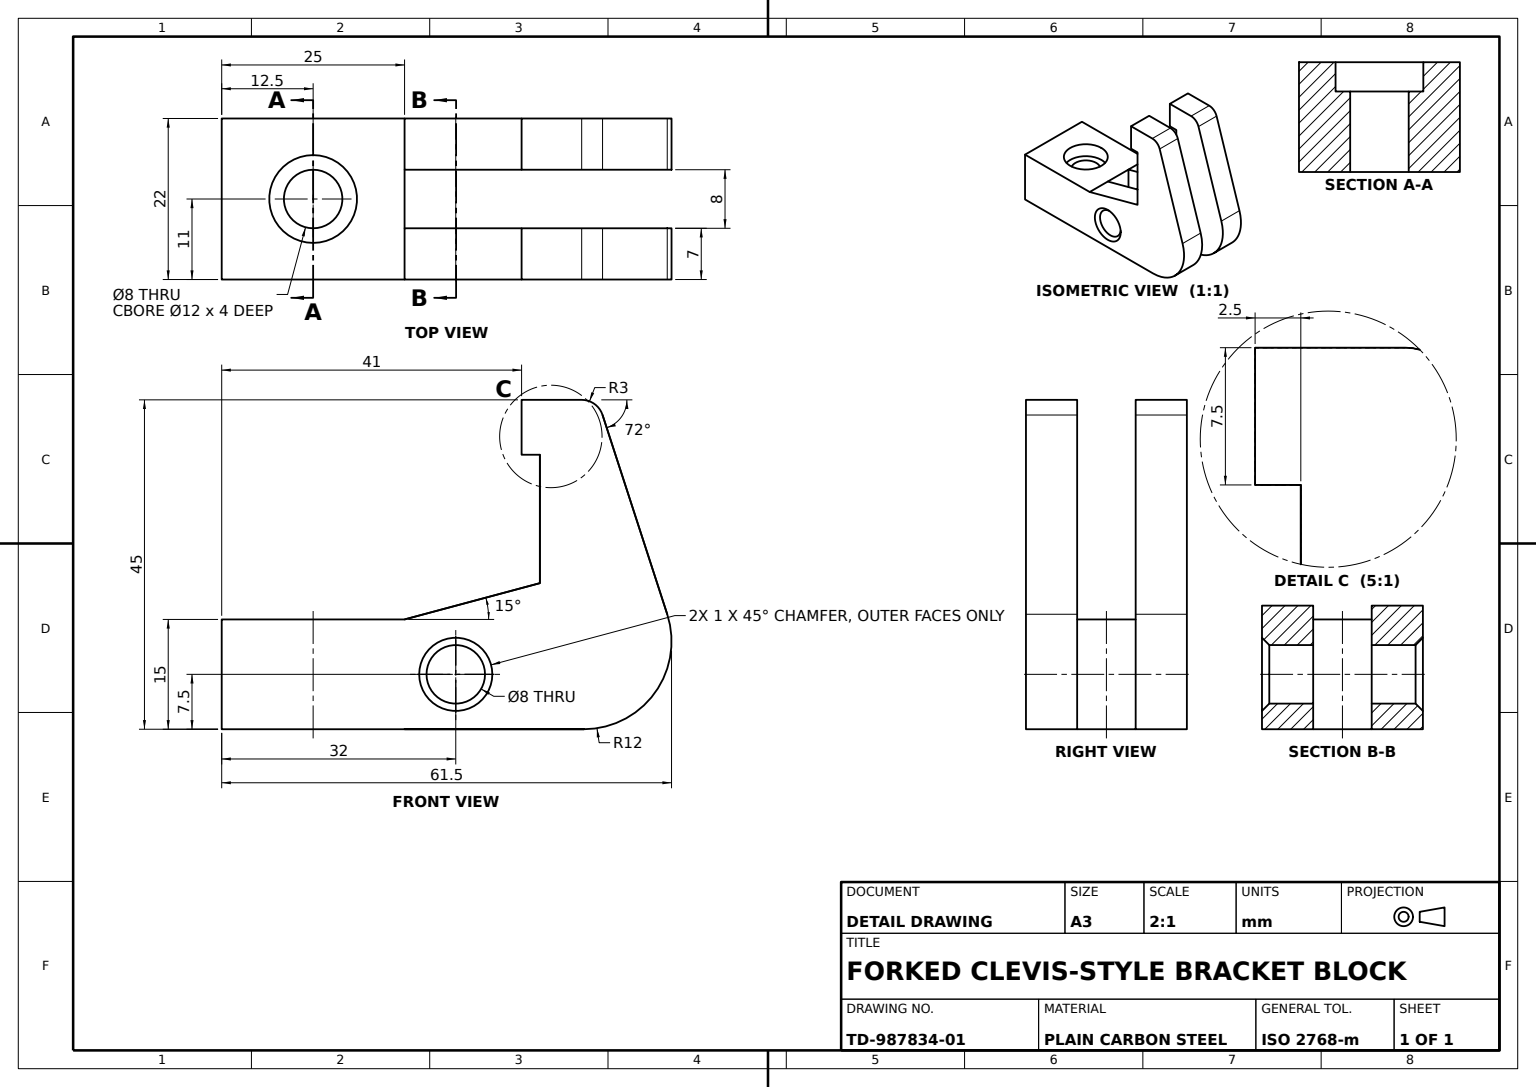
SolidWorks part; units mm, degrees
material "Plain Carbon Steel"
ref_plane "Front Plane" through (0, 0, 0) normal (0, 0, 1) x (1, 0, 0)
ref_plane "Top Plane" through (0, 0, 0) normal (0, 1, 0) x (1, 0, 0)
ref_plane "Right Plane" through (0, 0, 0) normal (1, 0, 0) x (0, 0, -1)
sketch "Bracket Profile Sketch" plane through (0, 0, 0) normal (0, 0, 1) x (1, 0, 0)
  line L0 (0, 0) -> (32, 0)
  line L1 (0, 0) -> (0, 15)
  line L2 (0, 15) -> (25, 15)
  line L3 (25, 15) -> (54.9393, 15) construction
  line L4 (25, 15) -> (43.5, 19.9571)
  line L5 (32, 0) -> (49.5, 0)
  line L6 (61.5, 0.3901) -> (61.5, 45) construction
  line L7 (43.5, 19.9571) -> (43.5, 37.5)
  line L8 (43.5, 37.5) -> (41, 37.5)
  line L9 (41, 37.5) -> (41, 45)
  line L10 (41, 45) -> (49.2156, 45)
  line L12 (52.0687, 42.9271) -> (60.9127, 15.7082)
  arc A1 (49.2156, 45) -> (52.0687, 42.9271) centre (49.2156, 42) cw
  arc A2 (49.5, 0) -> (60.9127, 15.7082) centre (49.5, 12) ccw
  dimension "D11" = 12
  dimension "D12" = 3
  dimension "D1" = 15
  dimension "D2" = 32
  dimension "D3" = 25
  dimension "D4" = 15
  dimension "D5" = 18
  dimension "D6" = 45
  dimension "D7" = 2.5
  dimension "D8" = 41
  dimension "D9" = 7.5
  dimension "D10" = 61.5
extrude "Bracket Body" add sketch "Bracket Profile Sketch" along normal mid plane 22
sketch "Fork Slot Sketch" plane through (0, 0, 0) normal (0, 1, 0) x (1, 0, 0)
  line L0 (25, -11) -> (25, 11) construction
  line L1 (25, 4) -> (61.5, 4)
  line L2 (25, 4) -> (25, -4)
  line L3 (25, -4) -> (61.5, -4)
  line L4 (61.5, 4) -> (61.5, -4)
  line L6 (61.5, -11) -> (61.5, 11) construction
  point P6 (25, 0)
  dimension "D1" = 8
extrude "Fork Slot 8mm" cut sketch "Fork Slot Sketch" along normal through all
hole_wizard "Mounting Hole CBore Ø8" positions "3DSketch1" profile "Sketch3" legacy end condition up to next
sketch3d "3DSketch1"
  line L0 (25, 15, 11) -> (0, 15, 11) construction
  line L3 (25, 15, -11) -> (0, 15, -11) construction
  point P0 (12.5, 15, 0)
  point P8 (12.5, 15, 11)
  dimension "D1" = 11
sketch "Sketch3" plane through (12.5, 15, 0) normal (1, 0, 0) x (0, 0, 1)
  line L0 (0, 0) -> (0, 15)
  line L1 (0, 15) -> (4, 15)
  line L2 (4, 15) -> (4, 4)
  line L3 (4, 4) -> (6, 4)
  line L4 (6, 4) -> (6, 0)
  line L5 (6, 0) -> (0, 0)
  line L6 (0, 110) -> (0, -10) construction
  dimension "Diameter" = 8
  dimension "Depth" = 15
  dimension "C-Bore Diameter" = 12
  dimension "C-Bore Depth" = 4
sketch "Cross Hole Sketch" plane through (0, 0, 11) normal (0, 0, 1) x (1, 0, 0)
  line L0 (0, 0) -> (49.5, 0) construction
  circle A0 centre (32, 7.5) radius 4
  dimension "D1" = 8
  dimension "D2" = 7.5
  dimension "D3" = 32
extrude "Cross Hole Ø8" cut sketch "Cross Hole Sketch" against normal through all
chamfer "Cross Hole Chamfer 1mm" distance 1 angle 45 2 edges at (36, 7.5, -11) (36, 7.5, 11)
